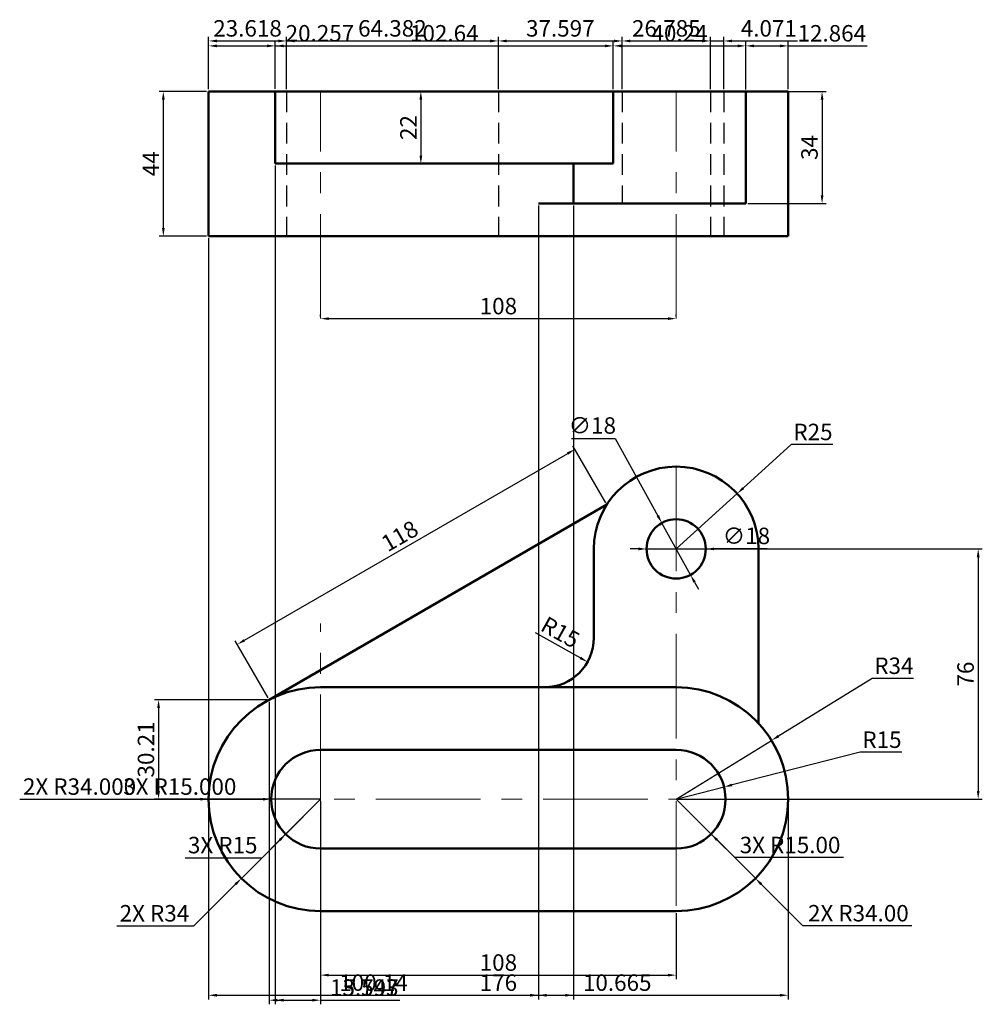
# Model space of a CAD drawing. Units: millimetres. Extents: x 1162 to 1454, y 1698 to 1997.
import ezdxf

# ---------------------------------------------------------------- set-up
doc = ezdxf.new("R2010")
doc.units = ezdxf.units.MM
doc.linetypes.add('CENTER', pattern=[50.8, 31.75, -6.35, 6.35, -6.35])
doc.linetypes.add('HIDDEN', pattern=[9.525, 6.35, -3.175])
for name, color, linetype, lineweight in [('M-CNTR', 1, 'CENTER', 18), ('M-DIMS', 2, 'Continuous', 25), ('M-HIDN', 3, 'HIDDEN', 25), ('M-OUTL', 7, 'Continuous', 50)]:
    doc.layers.add(name, color=color, linetype=linetype, lineweight=lineweight)
doc.styles.get("Standard").update_dxf_attribs({"font": 'arial.ttf'})
doc.dimstyles.new('ISO-25', dxfattribs={"dimtxt": 5, "dimasz": 2.5, "dimexe": 1.25, "dimexo": 0.625, "dimtad": 1, "dimtoh": 1, "dimdec": 0, "dimtxsty": 'Standard', "dimcen": 2.5, "dimadec": 0, "dimazin": 0, "dimtfac": 1, "dimtdec": 0, "dimtmove": 0, "dimatfit": 3, "dimfxl": 1, "dimarcsym": 0})

# ---------------------------------------------------------------- blocks, each defined once
blk = doc.blocks.new('*D1')
at = {"layer": 'Defpoints', "color": 0, "transparency": 16777216}
for p in [(1253.49, 1725.8), (1361.49, 1725.8), (1361.49, 1706.36)]:
    blk.add_point(p, dxfattribs=at)
at = {"layer": 'M-DIMS', "color": 0, "lineweight": -2, "transparency": 16777216}
for p, q in [((1253.49, 1725.18), (1253.49, 1705.11)), ((1361.49, 1725.18), (1361.49, 1705.11)), ((1255.99, 1706.36), (1358.99, 1706.36))]:
    blk.add_line(p, q, dxfattribs=at)
at = {"layer": 'M-DIMS', "color": 0, "transparency": 16777216}
for points in [[(1255.99, 1706.78), (1255.99, 1705.95), (1253.49, 1706.36)], [(1358.99, 1706.78), (1358.99, 1705.95), (1361.49, 1706.36)]]:
    blk.add_solid(points, dxfattribs=at)
at = {"layer": 'M-DIMS', "color": 0, "transparency": 16777216, "insert": (1307.49, 1709.54), "char_height": 5, "attachment_point": 5}
blk.add_mtext('108', dxfattribs=at)
blk = doc.blocks.new('*D2')
at = {"layer": 'Defpoints', "color": 0, "transparency": 16777216}
for p in [(1390.43, 1777.65), (1361.49, 1759.8)]:
    blk.add_point(p, dxfattribs=at)
at = {"layer": 'M-DIMS', "color": 0, "lineweight": -2, "transparency": 16777216}
for p, q in [((1421.01, 1796.5), (1392.56, 1778.96)), ((1433.56, 1796.5), (1421.01, 1796.5)), ((1361.49, 1759.8), (1390.43, 1777.65))]:
    blk.add_line(p, q, dxfattribs=at)
at = {"layer": 'M-DIMS', "color": 0, "transparency": 16777216}
blk.add_solid([(1392.34, 1779.31), (1392.78, 1778.6), (1390.43, 1777.65)], dxfattribs=at)
at = {"layer": 'M-DIMS', "color": 0, "transparency": 16777216, "insert": (1427.6, 1799.68), "char_height": 5, "attachment_point": 5}
blk.add_mtext('R34', dxfattribs=at)
blk = doc.blocks.new('*D3')
at = {"layer": 'Defpoints', "color": 0, "transparency": 16777216}
for p in [(1380, 1852.61), (1361.49, 1835.8)]:
    blk.add_point(p, dxfattribs=at)
at = {"layer": 'M-DIMS', "color": 0, "lineweight": -2, "transparency": 16777216}
for p, q in [((1396.41, 1867.51), (1381.85, 1854.29)), ((1409.02, 1867.51), (1396.41, 1867.51)), ((1361.49, 1835.8), (1380, 1852.61))]:
    blk.add_line(p, q, dxfattribs=at)
at = {"layer": 'M-DIMS', "color": 0, "transparency": 16777216}
blk.add_solid([(1381.57, 1854.6), (1382.13, 1853.98), (1380, 1852.61)], dxfattribs=at)
at = {"layer": 'M-DIMS', "color": 0, "transparency": 16777216, "insert": (1403.03, 1870.69), "char_height": 5, "attachment_point": 5}
blk.add_mtext('R25', dxfattribs=at)
blk = doc.blocks.new('*D4')
at = {"layer": 'Defpoints', "color": 0, "transparency": 16777216}
for p in [(1357.13, 1843.68), (1365.84, 1827.93)]:
    blk.add_point(p, dxfattribs=at)
at = {"layer": 'M-DIMS', "color": 0, "lineweight": -2, "transparency": 16777216}
for p, q in [((1329.71, 1869.33), (1342.95, 1869.33)), ((1342.95, 1869.33), (1355.92, 1845.87)), ((1365.84, 1827.93), (1357.13, 1843.68)), ((1367.05, 1825.74), (1368.26, 1823.55))]:
    blk.add_line(p, q, dxfattribs=at)
at = {"layer": 'M-DIMS', "color": 0, "transparency": 16777216}
for points in [[(1356.29, 1846.07), (1355.56, 1845.67), (1357.13, 1843.68)], [(1367.42, 1825.94), (1366.69, 1825.54), (1365.84, 1827.93)]]:
    blk.add_solid(points, dxfattribs=at)
at = {"layer": 'M-DIMS', "color": 0, "transparency": 16777216, "insert": (1336.02, 1872.65), "char_height": 5, "attachment_point": 5}
blk.add_mtext('∅18', dxfattribs=at)
blk = doc.blocks.new('*D5')
at = {"layer": 'Defpoints', "color": 0, "transparency": 16777216}
for p in [(1376.02, 1763.51), (1361.49, 1759.8)]:
    blk.add_point(p, dxfattribs=at)
at = {"layer": 'M-DIMS', "color": 0, "lineweight": -2, "transparency": 16777216}
for p, q in [((1417.37, 1774.04), (1378.45, 1764.12)), ((1429.98, 1774.04), (1417.37, 1774.04)), ((1361.49, 1759.8), (1376.02, 1763.51))]:
    blk.add_line(p, q, dxfattribs=at)
at = {"layer": 'M-DIMS', "color": 0, "transparency": 16777216}
blk.add_solid([(1378.34, 1764.53), (1378.55, 1763.72), (1376.02, 1763.51)], dxfattribs=at)
at = {"layer": 'M-DIMS', "color": 0, "transparency": 16777216, "insert": (1423.98, 1777.22), "char_height": 5, "attachment_point": 5}
blk.add_mtext('R15', dxfattribs=at)
blk = doc.blocks.new('*D6')
at = {"layer": 'Defpoints', "color": 0, "transparency": 16777216}
for p in [(1321.49, 1808.8), (1334.58, 1801.48)]:
    blk.add_point(p, dxfattribs=at)
at = {"layer": 'M-DIMS', "color": 0, "lineweight": -2, "transparency": 16777216}
blk.add_line((1318.66, 1810.38), (1332.4, 1802.7), dxfattribs=at)
at = {"layer": 'M-DIMS', "color": 0, "transparency": 16777216}
blk.add_solid([(1332.6, 1803.07), (1332.19, 1802.34), (1334.58, 1801.48)], dxfattribs=at)
at = {"layer": 'M-DIMS', "color": 0, "transparency": 16777216, "insert": (1325.99, 1809.93), "char_height": 5, "attachment_point": 5, "rotation": 330.782}
blk.add_mtext('R15', dxfattribs=at)
blk = doc.blocks.new('*D7')
at = {"layer": 'Defpoints', "color": 0, "transparency": 16777216}
for p in [(1330.71, 1866.05), (1340.41, 1849.25), (1237.89, 1790.02)]:
    blk.add_point(p, dxfattribs=at)
at = {"layer": 'M-DIMS', "color": 0, "lineweight": -2, "transparency": 16777216}
for p, q in [((1340.1, 1849.79), (1330.08, 1867.13)), ((1230.35, 1808.06), (1328.54, 1864.8)), ((1237.58, 1790.56), (1227.56, 1807.89))]:
    blk.add_line(p, q, dxfattribs=at)
at = {"layer": 'M-DIMS', "color": 0, "transparency": 16777216}
for points in [[(1328.34, 1865.16), (1328.75, 1864.44), (1330.71, 1866.05)], [(1230.14, 1808.42), (1230.56, 1807.7), (1228.19, 1806.81)]]:
    blk.add_solid(points, dxfattribs=at)
at = {"layer": 'M-DIMS', "color": 0, "transparency": 16777216, "insert": (1277.86, 1839.18), "char_height": 5, "attachment_point": 5, "rotation": 30.0195}
blk.add_mtext('118', dxfattribs=at)
blk = doc.blocks.new('*D8')
at = {"layer": 'Defpoints', "color": 0, "transparency": 16777216}
for p in [(1361.49, 1835.8), (1361.49, 1759.8), (1453.21, 1759.8)]:
    blk.add_point(p, dxfattribs=at)
at = {"layer": 'M-DIMS', "color": 0, "lineweight": -2, "transparency": 16777216}
for p, q in [((1362.11, 1835.8), (1454.46, 1835.8)), ((1453.21, 1833.3), (1453.21, 1762.3)), ((1362.11, 1759.8), (1454.46, 1759.8))]:
    blk.add_line(p, q, dxfattribs=at)
at = {"layer": 'M-DIMS', "color": 0, "transparency": 16777216}
for points in [[(1452.79, 1833.3), (1453.63, 1833.3), (1453.21, 1835.8)], [(1452.79, 1762.3), (1453.63, 1762.3), (1453.21, 1759.8)]]:
    blk.add_solid(points, dxfattribs=at)
at = {"layer": 'M-DIMS', "color": 0, "transparency": 16777216, "insert": (1450.03, 1797.8), "char_height": 5, "attachment_point": 5, "rotation": 90}
blk.add_mtext('76', dxfattribs=at)
blk = doc.blocks.new('*D9')
at = {"layer": 'Defpoints', "color": 0, "transparency": 16777216}
for p in [(1253.49, 1905.75), (1361.49, 1905.75), (1361.49, 1905.75)]:
    blk.add_point(p, dxfattribs=at)
at = {"layer": 'M-DIMS', "color": 0, "lineweight": -2, "transparency": 16777216}
for p, q in [((1253.49, 1906.37), (1253.49, 1907)), ((1255.99, 1905.75), (1358.99, 1905.75)), ((1361.49, 1906.37), (1361.49, 1907))]:
    blk.add_line(p, q, dxfattribs=at)
at = {"layer": 'M-DIMS', "color": 0, "transparency": 16777216}
for points in [[(1255.99, 1906.16), (1255.99, 1905.33), (1253.49, 1905.75)], [(1358.99, 1906.16), (1358.99, 1905.33), (1361.49, 1905.75)]]:
    blk.add_solid(points, dxfattribs=at)
at = {"layer": 'M-DIMS', "color": 0, "transparency": 16777216, "insert": (1307.49, 1908.92), "char_height": 5, "attachment_point": 5}
blk.add_mtext('108', dxfattribs=at)
blk = doc.blocks.new('*D10')
at = {"layer": 'Defpoints', "color": 0, "transparency": 16777216}
for p in [(1219.49, 1974.79), (1205.73, 1930.79), (1219.49, 1930.79)]:
    blk.add_point(p, dxfattribs=at)
at = {"layer": 'M-DIMS', "color": 0, "lineweight": -2, "transparency": 16777216}
for p, q in [((1218.86, 1974.79), (1204.48, 1974.79)), ((1205.73, 1972.29), (1205.73, 1933.29)), ((1218.86, 1930.79), (1204.48, 1930.79))]:
    blk.add_line(p, q, dxfattribs=at)
at = {"layer": 'M-DIMS', "color": 0, "transparency": 16777216}
for points in [[(1205.32, 1972.29), (1206.15, 1972.29), (1205.73, 1974.79)], [(1205.32, 1933.29), (1206.15, 1933.29), (1205.73, 1930.79)]]:
    blk.add_solid(points, dxfattribs=at)
at = {"layer": 'M-DIMS', "color": 0, "transparency": 16777216, "insert": (1202.61, 1952.79), "char_height": 5, "attachment_point": 5, "rotation": 90}
blk.add_mtext('44', dxfattribs=at)
blk = doc.blocks.new('*D11')
at = {"layer": 'Defpoints', "color": 0, "transparency": 16777216}
for p in [(1307.49, 1974.79), (1283.94, 1952.79), (1307.49, 1952.79)]:
    blk.add_point(p, dxfattribs=at)
at = {"layer": 'M-DIMS', "color": 0, "lineweight": -2, "transparency": 16777216}
for p, q in [((1306.86, 1974.79), (1282.69, 1974.79)), ((1283.94, 1972.29), (1283.94, 1955.29)), ((1306.86, 1952.79), (1282.69, 1952.79))]:
    blk.add_line(p, q, dxfattribs=at)
at = {"layer": 'M-DIMS', "color": 0, "transparency": 16777216}
for points in [[(1283.52, 1972.29), (1284.36, 1972.29), (1283.94, 1974.79)], [(1283.52, 1955.29), (1284.36, 1955.29), (1283.94, 1952.79)]]:
    blk.add_solid(points, dxfattribs=at)
at = {"layer": 'M-DIMS', "color": 0, "transparency": 16777216, "insert": (1280.81, 1963.79), "char_height": 5, "attachment_point": 5, "rotation": 90}
blk.add_mtext('22', dxfattribs=at)
blk = doc.blocks.new('*D12')
at = {"layer": 'Defpoints', "color": 0, "transparency": 16777216}
for p in [(1382.62, 1974.73), (1382.62, 1940.73), (1405.8, 1940.73)]:
    blk.add_point(p, dxfattribs=at)
at = {"layer": 'M-DIMS', "color": 0, "lineweight": -2, "transparency": 16777216}
for p, q in [((1383.25, 1974.73), (1407.05, 1974.73)), ((1405.8, 1972.23), (1405.8, 1943.23)), ((1383.25, 1940.73), (1407.05, 1940.73))]:
    blk.add_line(p, q, dxfattribs=at)
at = {"layer": 'M-DIMS', "color": 0, "transparency": 16777216}
for points in [[(1405.38, 1972.23), (1406.22, 1972.23), (1405.8, 1974.73)], [(1405.38, 1943.23), (1406.22, 1943.23), (1405.8, 1940.73)]]:
    blk.add_solid(points, dxfattribs=at)
at = {"layer": 'M-DIMS', "color": 0, "transparency": 16777216, "insert": (1402.62, 1957.73), "char_height": 5, "attachment_point": 5, "rotation": 90}
blk.add_mtext('34', dxfattribs=at)
blk = doc.blocks.new('*D13')
at = {"layer": 'Defpoints', "color": 0, "transparency": 16777216}
for p in [(1239.74, 1988.59), (1219.49, 1974.79), (1239.74, 1974.89)]:
    blk.add_point(p, dxfattribs=at)
at = {"layer": 'M-DIMS', "color": 0, "lineweight": -2, "transparency": 16777216}
for p, q in [((1219.49, 1975.41), (1219.49, 1989.84)), ((1239.74, 1975.51), (1239.74, 1989.84)), ((1221.99, 1988.59), (1237.24, 1988.59)), ((1239.74, 1988.59), (1264.34, 1988.59))]:
    blk.add_line(p, q, dxfattribs=at)
at = {"layer": 'M-DIMS', "color": 0, "transparency": 16777216}
for points in [[(1221.99, 1989), (1221.99, 1988.17), (1219.49, 1988.59)], [(1237.24, 1989), (1237.24, 1988.17), (1239.74, 1988.59)]]:
    blk.add_solid(points, dxfattribs=at)
at = {"layer": 'M-DIMS', "color": 0, "transparency": 16777216, "insert": (1253.29, 1991.77), "char_height": 5, "attachment_point": 5}
blk.add_mtext('20.257', dxfattribs=at)
blk = doc.blocks.new('*D14')
at = {"layer": 'Defpoints', "color": 0, "transparency": 16777216}
for p in [(1342.38, 1988.59), (1239.74, 1974.89), (1342.38, 1974.79)]:
    blk.add_point(p, dxfattribs=at)
at = {"layer": 'M-DIMS', "color": 0, "lineweight": -2, "transparency": 16777216}
for p, q in [((1239.74, 1975.51), (1239.74, 1989.84)), ((1342.38, 1975.41), (1342.38, 1989.84)), ((1242.24, 1988.59), (1339.88, 1988.59))]:
    blk.add_line(p, q, dxfattribs=at)
at = {"layer": 'M-DIMS', "color": 0, "transparency": 16777216}
for points in [[(1242.24, 1989), (1242.24, 1988.17), (1239.74, 1988.59)], [(1339.88, 1989), (1339.88, 1988.17), (1342.38, 1988.59)]]:
    blk.add_solid(points, dxfattribs=at)
at = {"layer": 'M-DIMS', "color": 0, "transparency": 16777216, "insert": (1291.06, 1991.77), "char_height": 5, "attachment_point": 5}
blk.add_mtext('102.64', dxfattribs=at)
blk = doc.blocks.new('*D15')
at = {"layer": 'Defpoints', "color": 0, "transparency": 16777216}
for p in [(1382.62, 1988.59), (1342.38, 1974.79), (1382.62, 1974.73)]:
    blk.add_point(p, dxfattribs=at)
at = {"layer": 'M-DIMS', "color": 0, "lineweight": -2, "transparency": 16777216}
for p, q in [((1342.38, 1975.41), (1342.38, 1989.84)), ((1382.62, 1975.36), (1382.62, 1989.84)), ((1344.88, 1988.59), (1380.12, 1988.59))]:
    blk.add_line(p, q, dxfattribs=at)
at = {"layer": 'M-DIMS', "color": 0, "transparency": 16777216}
for points in [[(1344.88, 1989), (1344.88, 1988.17), (1342.38, 1988.59)], [(1380.12, 1989), (1380.12, 1988.17), (1382.62, 1988.59)]]:
    blk.add_solid(points, dxfattribs=at)
at = {"layer": 'M-DIMS', "color": 0, "transparency": 16777216, "insert": (1362.5, 1991.77), "char_height": 5, "attachment_point": 5}
blk.add_mtext('40.24', dxfattribs=at)
blk = doc.blocks.new('*D16')
at = {"layer": 'Defpoints', "color": 0, "transparency": 16777216}
for p in [(1395.49, 1988.59), (1382.62, 1974.73), (1395.49, 1974.79)]:
    blk.add_point(p, dxfattribs=at)
at = {"layer": 'M-DIMS', "color": 0, "lineweight": -2, "transparency": 16777216}
for p, q in [((1382.62, 1975.36), (1382.62, 1989.84)), ((1395.49, 1975.41), (1395.49, 1989.84)), ((1385.12, 1988.59), (1392.99, 1988.59)), ((1395.49, 1988.59), (1419.5, 1988.59))]:
    blk.add_line(p, q, dxfattribs=at)
at = {"layer": 'M-DIMS', "color": 0, "transparency": 16777216}
for points in [[(1385.12, 1989), (1385.12, 1988.17), (1382.62, 1988.59)], [(1392.99, 1989), (1392.99, 1988.17), (1395.49, 1988.59)]]:
    blk.add_solid(points, dxfattribs=at)
at = {"layer": 'M-DIMS', "color": 0, "transparency": 16777216, "insert": (1408.75, 1991.77), "char_height": 5, "attachment_point": 5}
blk.add_mtext('12.864', dxfattribs=at)
blk = doc.blocks.new('*D17')
at = {"layer": 'Defpoints', "color": 0, "transparency": 16777216}
for p in [(1319.63, 1940.73), (1219.49, 1930.79), (1319.63, 1700.25)]:
    blk.add_point(p, dxfattribs=at)
at = {"layer": 'M-DIMS', "color": 0, "lineweight": -2, "transparency": 16777216}
for p, q in [((1319.63, 1940.11), (1319.63, 1699)), ((1219.49, 1930.16), (1219.49, 1699)), ((1221.99, 1700.25), (1317.13, 1700.25))]:
    blk.add_line(p, q, dxfattribs=at)
at = {"layer": 'M-DIMS', "color": 0, "transparency": 16777216}
for points in [[(1221.99, 1700.67), (1221.99, 1699.83), (1219.49, 1700.25)], [(1317.13, 1700.67), (1317.13, 1699.83), (1319.63, 1700.25)]]:
    blk.add_solid(points, dxfattribs=at)
at = {"layer": 'M-DIMS', "color": 0, "transparency": 16777216, "insert": (1269.56, 1703.43), "char_height": 5, "attachment_point": 5}
blk.add_mtext('100.14', dxfattribs=at)
blk = doc.blocks.new('*D18')
at = {"layer": 'Defpoints', "color": 0, "transparency": 16777216}
for p in [(1319.63, 1940.73), (1330.3, 1940.73), (1330.3, 1700.25)]:
    blk.add_point(p, dxfattribs=at)
at = {"layer": 'M-DIMS', "color": 0, "lineweight": -2, "transparency": 16777216}
for p, q in [((1319.63, 1940.11), (1319.63, 1699)), ((1330.3, 1940.11), (1330.3, 1699)), ((1322.13, 1700.25), (1327.8, 1700.25)), ((1330.3, 1700.25), (1354.37, 1700.25))]:
    blk.add_line(p, q, dxfattribs=at)
at = {"layer": 'M-DIMS', "color": 0, "transparency": 16777216}
for points in [[(1322.13, 1700.67), (1322.13, 1699.83), (1319.63, 1700.25)], [(1327.8, 1700.67), (1327.8, 1699.83), (1330.3, 1700.25)]]:
    blk.add_solid(points, dxfattribs=at)
at = {"layer": 'M-DIMS', "color": 0, "transparency": 16777216, "insert": (1343.58, 1703.43), "char_height": 5, "attachment_point": 5}
blk.add_mtext('10.665', dxfattribs=at)
blk = doc.blocks.new('*D19')
at = {"layer": 'Defpoints', "color": 0, "transparency": 16777216}
for p in [(1219.49, 1759.8), (1395.49, 1759.8), (1395.49, 1700.25)]:
    blk.add_point(p, dxfattribs=at)
at = {"layer": 'M-DIMS', "color": 0, "lineweight": -2, "transparency": 16777216}
for p, q in [((1219.49, 1759.18), (1219.49, 1699)), ((1395.49, 1759.18), (1395.49, 1699)), ((1221.99, 1700.25), (1392.99, 1700.25))]:
    blk.add_line(p, q, dxfattribs=at)
at = {"layer": 'M-DIMS', "color": 0, "transparency": 16777216}
for points in [[(1221.99, 1700.67), (1221.99, 1699.83), (1219.49, 1700.25)], [(1392.99, 1700.67), (1392.99, 1699.83), (1395.49, 1700.25)]]:
    blk.add_solid(points, dxfattribs=at)
at = {"layer": 'M-DIMS', "color": 0, "transparency": 16777216, "insert": (1307.49, 1703.43), "char_height": 5, "attachment_point": 5}
blk.add_mtext('176', dxfattribs=at)
blk = doc.blocks.new('*D20')
at = {"layer": 'Defpoints', "color": 0, "transparency": 16777216}
for p in [(1253.49, 1759.8), (1229.45, 1735.75)]:
    blk.add_point(p, dxfattribs=at)
at = {"layer": 'M-DIMS', "color": 0, "lineweight": -2, "transparency": 16777216}
for p, q in [((1253.49, 1759.8), (1229.45, 1735.75)), ((1215.03, 1721.32), (1227.69, 1733.99)), ((1191.65, 1721.32), (1215.03, 1721.32))]:
    blk.add_line(p, q, dxfattribs=at)
at = {"layer": 'M-DIMS', "color": 0, "transparency": 16777216}
blk.add_solid([(1227.39, 1734.28), (1227.98, 1733.69), (1229.45, 1735.75)], dxfattribs=at)
at = {"layer": 'M-DIMS', "color": 0, "transparency": 16777216, "insert": (1203.03, 1724.5), "char_height": 5, "attachment_point": 5}
blk.add_mtext('2X R34', dxfattribs=at)
blk = doc.blocks.new('*D21')
at = {"layer": 'Defpoints', "color": 0, "transparency": 16777216}
for p in [(1253.49, 1759.8), (1242.89, 1749.19)]:
    blk.add_point(p, dxfattribs=at)
at = {"layer": 'M-DIMS', "color": 0, "lineweight": -2, "transparency": 16777216}
for p, q in [((1253.49, 1759.8), (1242.89, 1749.19)), ((1235.75, 1742.03), (1241.12, 1747.42)), ((1212.4, 1742.03), (1235.75, 1742.03))]:
    blk.add_line(p, q, dxfattribs=at)
at = {"layer": 'M-DIMS', "color": 0, "transparency": 16777216}
blk.add_solid([(1240.83, 1747.71), (1241.42, 1747.13), (1242.89, 1749.19)], dxfattribs=at)
at = {"layer": 'M-DIMS', "color": 0, "transparency": 16777216, "insert": (1223.76, 1745.21), "char_height": 5, "attachment_point": 5}
blk.add_mtext('3X R15', dxfattribs=at)
blk = doc.blocks.new('*D22')
at = {"layer": 'Defpoints', "color": 0, "transparency": 16777216}
for p in [(1352.49, 1835.8), (1370.49, 1835.8)]:
    blk.add_point(p, dxfattribs=at)
at = {"layer": 'M-DIMS', "color": 0, "lineweight": -2, "transparency": 16777216}
for p, q in [((1349.99, 1835.8), (1347.49, 1835.8)), ((1352.49, 1835.8), (1370.49, 1835.8)), ((1375.89, 1835.8), (1372.99, 1835.8)), ((1389.12, 1835.8), (1375.89, 1835.8))]:
    blk.add_line(p, q, dxfattribs=at)
at = {"layer": 'M-DIMS', "color": 0, "transparency": 16777216}
for points in [[(1349.99, 1836.22), (1349.99, 1835.39), (1352.49, 1835.8)], [(1372.99, 1836.22), (1372.99, 1835.39), (1370.49, 1835.8)]]:
    blk.add_solid(points, dxfattribs=at)
at = {"layer": 'M-DIMS', "color": 0, "transparency": 16777216, "insert": (1382.82, 1839.12), "char_height": 5, "attachment_point": 5}
blk.add_mtext('∅18', dxfattribs=at)
blk = doc.blocks.new('*D23')
at = {"layer": 'Defpoints', "color": 0, "transparency": 16777216}
for p in [(1237.89, 1790.02), (1204.29, 1759.8), (1253.49, 1759.8)]:
    blk.add_point(p, dxfattribs=at)
at = {"layer": 'M-DIMS', "color": 0, "lineweight": -2, "transparency": 16777216}
for p, q in [((1237.27, 1790.02), (1203.04, 1790.02)), ((1204.29, 1787.52), (1204.29, 1762.3)), ((1252.86, 1759.8), (1203.04, 1759.8))]:
    blk.add_line(p, q, dxfattribs=at)
at = {"layer": 'M-DIMS', "color": 0, "transparency": 16777216}
for points in [[(1203.87, 1787.52), (1204.7, 1787.52), (1204.29, 1790.02)], [(1203.87, 1762.3), (1204.7, 1762.3), (1204.29, 1759.8)]]:
    blk.add_solid(points, dxfattribs=at)
at = {"layer": 'M-DIMS', "color": 0, "transparency": 16777216, "insert": (1201.11, 1774.91), "char_height": 5, "attachment_point": 5, "rotation": 90}
blk.add_mtext('30.21', dxfattribs=at)
blk = doc.blocks.new('*D24')
at = {"layer": 'Defpoints', "color": 0, "transparency": 16777216}
for p in [(1237.89, 1790.02), (1253.49, 1759.8), (1253.49, 1698.75)]:
    blk.add_point(p, dxfattribs=at)
at = {"layer": 'M-DIMS', "color": 0, "lineweight": -2, "transparency": 16777216}
for p, q in [((1237.89, 1789.39), (1237.89, 1697.5)), ((1253.49, 1759.18), (1253.49, 1697.5)), ((1240.39, 1698.75), (1250.99, 1698.75)), ((1253.49, 1698.75), (1277.52, 1698.75))]:
    blk.add_line(p, q, dxfattribs=at)
at = {"layer": 'M-DIMS', "color": 0, "transparency": 16777216}
for points in [[(1240.39, 1699.17), (1240.39, 1698.33), (1237.89, 1698.75)], [(1250.99, 1699.17), (1250.99, 1698.33), (1253.49, 1698.75)]]:
    blk.add_solid(points, dxfattribs=at)
at = {"layer": 'M-DIMS', "color": 0, "transparency": 16777216, "insert": (1266.76, 1701.93), "char_height": 5, "attachment_point": 5}
blk.add_mtext('15.597', dxfattribs=at)
blk = doc.blocks.new('*D25')
at = {"layer": 'Defpoints', "color": 0, "transparency": 16777216}
for p in [(1239.74, 1952.89), (1253.49, 1759.8), (1253.49, 1698.75)]:
    blk.add_point(p, dxfattribs=at)
at = {"layer": 'M-DIMS', "color": 0, "lineweight": -2, "transparency": 16777216}
for p, q in [((1239.74, 1952.26), (1239.74, 1697.5)), ((1253.49, 1759.18), (1253.49, 1697.5)), ((1242.24, 1698.75), (1250.99, 1698.75)), ((1253.49, 1698.75), (1277.52, 1698.75))]:
    blk.add_line(p, q, dxfattribs=at)
at = {"layer": 'M-DIMS', "color": 0, "transparency": 16777216}
for points in [[(1242.24, 1699.17), (1242.24, 1698.33), (1239.74, 1698.75)], [(1250.99, 1699.17), (1250.99, 1698.33), (1253.49, 1698.75)]]:
    blk.add_solid(points, dxfattribs=at)
at = {"layer": 'M-DIMS', "color": 0, "transparency": 16777216, "insert": (1266.76, 1701.93), "char_height": 5, "attachment_point": 5}
blk.add_mtext('13.743', dxfattribs=at)
blk = doc.blocks.new('*D26')
at = {"layer": 'Defpoints', "color": 0, "transparency": 16777216}
for p in [(1361.49, 1759.8), (1385.53, 1735.77)]:
    blk.add_point(p, dxfattribs=at)
at = {"layer": 'M-DIMS', "color": 0, "lineweight": -2, "transparency": 16777216}
for p, q in [((1361.49, 1759.8), (1385.53, 1735.77)), ((1399.96, 1721.34), (1387.3, 1734)), ((1433.06, 1721.34), (1399.96, 1721.34))]:
    blk.add_line(p, q, dxfattribs=at)
at = {"layer": 'M-DIMS', "color": 0, "transparency": 16777216}
blk.add_solid([(1387.6, 1734.29), (1387.01, 1733.7), (1385.53, 1735.77)], dxfattribs=at)
at = {"layer": 'M-DIMS', "color": 0, "transparency": 16777216, "insert": (1416.82, 1724.52), "char_height": 5, "attachment_point": 5}
blk.add_mtext('2X R34.00', dxfattribs=at)
blk = doc.blocks.new('*D27')
at = {"layer": 'Defpoints', "color": 0, "transparency": 16777216}
for p in [(1361.49, 1759.8), (1372.1, 1749.2)]:
    blk.add_point(p, dxfattribs=at)
at = {"layer": 'M-DIMS', "color": 0, "lineweight": -2, "transparency": 16777216}
for p, q in [((1361.49, 1759.8), (1372.1, 1749.2)), ((1379.25, 1742.06), (1373.87, 1747.43)), ((1412.26, 1742.06), (1379.25, 1742.06))]:
    blk.add_line(p, q, dxfattribs=at)
at = {"layer": 'M-DIMS', "color": 0, "transparency": 16777216}
blk.add_solid([(1374.16, 1747.73), (1373.57, 1747.14), (1372.1, 1749.2)], dxfattribs=at)
at = {"layer": 'M-DIMS', "color": 0, "transparency": 16777216, "insert": (1396.07, 1745.24), "char_height": 5, "attachment_point": 5}
blk.add_mtext('3X R15.00', dxfattribs=at)
blk = doc.blocks.new('*D28')
at = {"layer": 'Defpoints', "color": 0, "transparency": 16777216}
for p in [(1243.11, 1990.09), (1219.49, 1974.79), (1243.11, 1974.79)]:
    blk.add_point(p, dxfattribs=at)
at = {"layer": 'M-DIMS', "color": 0, "lineweight": -2, "transparency": 16777216}
for p, q in [((1219.49, 1975.41), (1219.49, 1991.34)), ((1221.99, 1990.09), (1240.61, 1990.09)), ((1243.11, 1975.41), (1243.11, 1991.34))]:
    blk.add_line(p, q, dxfattribs=at)
at = {"layer": 'M-DIMS', "color": 0, "transparency": 16777216}
for points in [[(1221.99, 1990.5), (1221.99, 1989.67), (1219.49, 1990.09)], [(1240.61, 1990.5), (1240.61, 1989.67), (1243.11, 1990.09)]]:
    blk.add_solid(points, dxfattribs=at)
at = {"layer": 'M-DIMS', "color": 0, "transparency": 16777216, "insert": (1231.3, 1993.27), "char_height": 5, "attachment_point": 5}
blk.add_mtext('23.618', dxfattribs=at)
blk = doc.blocks.new('*D29')
at = {"layer": 'Defpoints', "color": 0, "transparency": 16777216}
for p in [(1307.49, 1990.09), (1243.11, 1974.79), (1307.49, 1974.79)]:
    blk.add_point(p, dxfattribs=at)
at = {"layer": 'M-DIMS', "color": 0, "lineweight": -2, "transparency": 16777216}
for p, q in [((1243.11, 1975.41), (1243.11, 1991.34)), ((1245.61, 1990.09), (1304.99, 1990.09)), ((1307.49, 1975.41), (1307.49, 1991.34))]:
    blk.add_line(p, q, dxfattribs=at)
at = {"layer": 'M-DIMS', "color": 0, "transparency": 16777216}
for points in [[(1245.61, 1990.5), (1245.61, 1989.67), (1243.11, 1990.09)], [(1304.99, 1990.5), (1304.99, 1989.67), (1307.49, 1990.09)]]:
    blk.add_solid(points, dxfattribs=at)
at = {"layer": 'M-DIMS', "color": 0, "transparency": 16777216, "insert": (1275.3, 1993.27), "char_height": 5, "attachment_point": 5}
blk.add_mtext('64.382', dxfattribs=at)
blk = doc.blocks.new('*D30')
at = {"layer": 'Defpoints', "color": 0, "transparency": 16777216}
for p in [(1345.08, 1990.09), (1307.49, 1974.79), (1345.08, 1974.79)]:
    blk.add_point(p, dxfattribs=at)
at = {"layer": 'M-DIMS', "color": 0, "lineweight": -2, "transparency": 16777216}
for p, q in [((1307.49, 1975.41), (1307.49, 1991.34)), ((1309.99, 1990.09), (1342.58, 1990.09)), ((1345.08, 1975.41), (1345.08, 1991.34))]:
    blk.add_line(p, q, dxfattribs=at)
at = {"layer": 'M-DIMS', "color": 0, "transparency": 16777216}
for points in [[(1309.99, 1990.5), (1309.99, 1989.67), (1307.49, 1990.09)], [(1342.58, 1990.5), (1342.58, 1989.67), (1345.08, 1990.09)]]:
    blk.add_solid(points, dxfattribs=at)
at = {"layer": 'M-DIMS', "color": 0, "transparency": 16777216, "insert": (1326.29, 1993.27), "char_height": 5, "attachment_point": 5}
blk.add_mtext('37.597', dxfattribs=at)
blk = doc.blocks.new('*D31')
at = {"layer": 'Defpoints', "color": 0, "transparency": 16777216}
for p in [(1371.87, 1990.09), (1345.08, 1974.79), (1371.87, 1974.79)]:
    blk.add_point(p, dxfattribs=at)
at = {"layer": 'M-DIMS', "color": 0, "lineweight": -2, "transparency": 16777216}
for p, q in [((1345.08, 1975.41), (1345.08, 1991.34)), ((1347.58, 1990.09), (1369.37, 1990.09)), ((1371.87, 1975.41), (1371.87, 1991.34))]:
    blk.add_line(p, q, dxfattribs=at)
at = {"layer": 'M-DIMS', "color": 0, "transparency": 16777216}
for points in [[(1347.58, 1990.5), (1347.58, 1989.67), (1345.08, 1990.09)], [(1369.37, 1990.5), (1369.37, 1989.67), (1371.87, 1990.09)]]:
    blk.add_solid(points, dxfattribs=at)
at = {"layer": 'M-DIMS', "color": 0, "transparency": 16777216, "insert": (1358.48, 1993.27), "char_height": 5, "attachment_point": 5}
blk.add_mtext('26.785', dxfattribs=at)
blk = doc.blocks.new('*D32')
at = {"layer": 'Defpoints', "color": 0, "transparency": 16777216}
for p in [(1375.94, 1990.09), (1371.87, 1974.79), (1375.94, 1974.79)]:
    blk.add_point(p, dxfattribs=at)
at = {"layer": 'M-DIMS', "color": 0, "lineweight": -2, "transparency": 16777216}
for p, q in [((1369.37, 1990.09), (1366.87, 1990.09)), ((1371.87, 1975.41), (1371.87, 1991.34)), ((1371.87, 1990.09), (1375.94, 1990.09)), ((1375.94, 1975.41), (1375.94, 1991.34)), ((1378.44, 1990.09), (1398.3, 1990.09))]:
    blk.add_line(p, q, dxfattribs=at)
at = {"layer": 'M-DIMS', "color": 0, "transparency": 16777216}
for points in [[(1369.37, 1990.5), (1369.37, 1989.67), (1371.87, 1990.09)], [(1378.44, 1990.5), (1378.44, 1989.67), (1375.94, 1990.09)]]:
    blk.add_solid(points, dxfattribs=at)
at = {"layer": 'M-DIMS', "color": 0, "transparency": 16777216, "insert": (1389.62, 1993.27), "char_height": 5, "attachment_point": 5}
blk.add_mtext('4.071', dxfattribs=at)
blk = doc.blocks.new('*D33')
at = {"layer": 'Defpoints', "color": 0, "transparency": 16777216}
for p in [(1219.49, 1759.8), (1253.49, 1759.8)]:
    blk.add_point(p, dxfattribs=at)
at = {"layer": 'M-DIMS', "color": 0, "lineweight": -2, "transparency": 16777216}
for p, q in [((1162.11, 1759.8), (1199.09, 1759.8)), ((1199.09, 1759.8), (1216.99, 1759.8)), ((1253.49, 1759.8), (1219.49, 1759.8))]:
    blk.add_line(p, q, dxfattribs=at)
at = {"layer": 'M-DIMS', "color": 0, "transparency": 16777216}
blk.add_solid([(1216.99, 1760.22), (1216.99, 1759.39), (1219.49, 1759.8)], dxfattribs=at)
at = {"layer": 'M-DIMS', "color": 0, "transparency": 16777216, "insert": (1180.29, 1762.98), "char_height": 5, "attachment_point": 5}
blk.add_mtext('2X R34.000', dxfattribs=at)
blk = doc.blocks.new('*D34')
at = {"layer": 'Defpoints', "color": 0, "transparency": 16777216}
for p in [(1238.49, 1759.8), (1253.49, 1759.8)]:
    blk.add_point(p, dxfattribs=at)
at = {"layer": 'M-DIMS', "color": 0, "lineweight": -2, "transparency": 16777216}
for p, q in [((1192.6, 1759.8), (1229.49, 1759.8)), ((1229.49, 1759.8), (1235.99, 1759.8)), ((1253.49, 1759.8), (1238.49, 1759.8))]:
    blk.add_line(p, q, dxfattribs=at)
at = {"layer": 'M-DIMS', "color": 0, "transparency": 16777216}
blk.add_solid([(1235.99, 1760.22), (1235.99, 1759.39), (1238.49, 1759.8)], dxfattribs=at)
at = {"layer": 'M-DIMS', "color": 0, "transparency": 16777216, "insert": (1210.73, 1762.98), "char_height": 5, "attachment_point": 5}
blk.add_mtext('3X R15.000', dxfattribs=at)

msp = doc.modelspace()

# ---------------------------------------------------------------- linework, layer by layer
at = {"layer": 'M-CNTR'}
for p, q in [((1253.4872, 1905.7464), (1253.4872, 1974.7868)), ((1361.4872, 1905.7464), (1361.4872, 1974.7868)), ((1361.4872, 1860.8035), (1361.4872, 1714.1546)), ((1253.4872, 1759.8035), (1253.4872, 1813.1897)), ((1219.4872, 1759.8035), (1395.4872, 1759.8035)), ((1253.4872, 1759.8035), (1253.4872, 1713.951))]:
    msp.add_line(p, q, dxfattribs=at)
at = {"layer": 'M-HIDN'}
for p, q in [((1243.105, 1974.7868), (1243.105, 1930.7868)), ((1243.105, 1974.7868), (1243.105, 1930.7868)), ((1243.105, 1974.7868), (1243.105, 1930.7868)), ((1307.4872, 1974.7868), (1307.4872, 1930.7868)), ((1345.0839, 1974.7868), (1345.0839, 1940.7321)), ((1371.8693, 1974.7868), (1371.8693, 1930.7868)), ((1375.94, 1974.7868), (1375.94, 1930.7868))]:
    msp.add_line(p, q, dxfattribs=at)
at = {"layer": 'M-OUTL'}
for p, q in [((1395.4872, 1974.7868), (1219.4872, 1974.7868)), ((1219.4872, 1974.7868), (1219.4872, 1930.7868)), ((1239.7445, 1974.8883), (1239.7445, 1952.8883)), ((1342.3807, 1952.8883), (1342.3807, 1974.7868)), ((1382.6231, 1974.7321), (1382.6231, 1940.7321)), ((1395.4872, 1930.7868), (1395.4872, 1974.7868)), ((1239.7445, 1952.8883), (1342.3807, 1952.8883)), ((1330.2957, 1940.7321), (1330.2957, 1952.8883)), ((1382.6231, 1940.7321), (1319.6312, 1940.7321)), ((1219.4872, 1930.7868), (1395.4872, 1930.7868)), ((1237.8905, 1790.0151), (1340.4134, 1849.2532)), ((1336.4872, 1835.8035), (1336.4872, 1808.8035)), ((1386.4872, 1835.8035), (1386.4872, 1782.8469)), ((1253.4872, 1793.8035), (1321.4872, 1793.8035)), ((1321.4872, 1793.8035), (1361.4872, 1793.8035)), ((1253.4872, 1774.8035), (1361.4872, 1774.8035)), ((1361.4872, 1744.8035), (1253.4872, 1744.8035)), ((1253.4872, 1725.8035), (1361.4872, 1725.8035))]:
    msp.add_line(p, q, dxfattribs=at)
msp.add_circle((1361.4872, 1835.8035), 9, dxfattribs=at)
for centre, radius, start, end in [((1361.4872, 1835.8035), 25, 0, 180), ((1321.4872, 1808.8035), 15, 270, 0), ((1253.4872, 1759.8035), 34, 90, 270), ((1361.4872, 1759.8035), 34, 270, 90), ((1253.4872, 1759.8035), 15, 90, 270), ((1361.4872, 1759.8035), 15, 270, 90)]:
    msp.add_arc(centre, radius, start, end, dxfattribs=at)

# ---------------------------------------------------------------- dimensions: what is measured, and where the dimension line sits
at = {"layer": 'M-DIMS'}
for base, p1, p2, override, picture, middle in [((1243.105, 1990.0883), (1219.4872, 1974.7868), (1243.105, 1974.7868), {"dimdec": 3, "dimlfac": 1, "dimrnd": 0, "dimzin": 0, "dimdsep": 46, "dimlunit": 2}, '*D28', (1231.2961, 1993.2679)), ((1239.7445, 1988.5883), (1219.4872, 1974.7868), (1239.7445, 1974.8883), {"dimdec": 3, "dimlfac": 1, "dimrnd": 0, "dimzin": 0, "dimdsep": 46, "dimlunit": 2}, '*D13', (1253.2908, 1991.7662)), ((1342.3807, 1988.5883), (1239.7445, 1974.8883), (1342.3807, 1974.7868), {"dimdec": 2, "dimlfac": 1, "dimrnd": 0, "dimzin": 0, "dimdsep": 46, "dimlunit": 2}, '*D14', (1291.0626, 1991.7662)), ((1307.4872, 1990.0883), (1243.105, 1974.7868), (1307.4872, 1974.7868), {"dimdec": 3, "dimlfac": 1, "dimrnd": 0, "dimzin": 0, "dimdsep": 46, "dimlunit": 2}, '*D29', (1275.2961, 1993.2679)), ((1345.0839, 1990.0883), (1307.4872, 1974.7868), (1345.0839, 1974.7868), {"dimdec": 3, "dimlfac": 1, "dimrnd": 0, "dimzin": 0, "dimdsep": 46, "dimlunit": 2}, '*D30', (1326.2855, 1993.2679)), ((1382.6231, 1988.5883), (1342.3807, 1974.7868), (1382.6231, 1974.7321), {"dimdec": 2, "dimlfac": 1, "dimrnd": 0, "dimzin": 0, "dimdsep": 46, "dimlunit": 2}, '*D15', (1362.5019, 1991.7662)), ((1371.8693, 1990.0883), (1345.0839, 1974.7868), (1371.8693, 1974.7868), {"dimdec": 3, "dimlfac": 1, "dimrnd": 0, "dimzin": 0, "dimdsep": 46, "dimlunit": 2}, '*D31', (1358.4766, 1993.2662)), ((1375.94, 1990.0883), (1371.8693, 1974.7868), (1375.94, 1974.7868), {"dimdec": 3, "dimlfac": 1, "dimrnd": 0, "dimzin": 0, "dimdsep": 46, "dimlunit": 2}, '*D32', (1389.6192, 1993.2662)), ((1395.4872, 1988.5883), (1382.6231, 1974.7321), (1395.4872, 1974.7868), {"dimdec": 3, "dimlfac": 1, "dimrnd": 0, "dimzin": 0, "dimdsep": 46, "dimlunit": 2}, '*D16', (1408.7452, 1991.7662)), ((1253.4872, 1698.751), (1239.7445, 1952.8883), (1253.4872, 1759.8035), {"dimdec": 3, "dimlfac": 1, "dimrnd": 0, "dimzin": 0, "dimdsep": 46, "dimlunit": 2}, '*D25', (1266.7554, 1701.9305)), ((1319.6312, 1700.251), (1219.4872, 1930.7868), (1319.6312, 1940.7321), {"dimdec": 2, "dimlfac": 1, "dimrnd": 0, "dimzin": 0, "dimdsep": 46, "dimlunit": 2}, '*D17', (1269.5592, 1703.4288)), ((1330.29571, 1700.25096), (1319.63117, 1940.73214), (1330.29571, 1940.73214), {"dimdec": 3, "dimlfac": 1, "dimrnd": 0, "dimzin": 0, "dimdsep": 46, "dimlunit": 2}, '*D18', (1343.58272, 1703.42882)), ((1361.4872, 1905.7464), (1253.4872, 1905.7464), (1361.4872, 1905.7464), {"dimclrd": 0, "dimclre": 0, "dimclrt": 0}, '*D9', (1307.4872, 1908.9242)), ((1253.4872, 1698.751), (1237.8905, 1790.0151), (1253.4872, 1759.8035), {"dimdec": 3, "dimlfac": 1, "dimrnd": 0, "dimzin": 0, "dimdsep": 46, "dimlunit": 2}, '*D24', (1266.7554, 1701.9288)), ((1395.4872, 1700.251), (1219.4872, 1759.8035), (1395.4872, 1759.8035), {"dimdec": 0, "dimlfac": 1, "dimrnd": 0, "dimzin": 0, "dimdsep": 46, "dimlunit": 2}, '*D19', (1307.4872, 1703.4288)), ((1361.4872, 1706.3639), (1253.4872, 1725.8035), (1361.4872, 1725.8035), {"dimclrd": 0, "dimclre": 0, "dimclrt": 0}, '*D1', (1307.4872, 1709.5418))]:
    dim = msp.add_linear_dim(base=base, p1=p1, p2=p2, dimstyle='ISO-25', override=override, dxfattribs=at)
    dim.commit()
    dim.dimension.update_dxf_attribs({"geometry": picture, "text_midpoint": middle})
for base, p1, p2, override, picture, middle in [((1205.7337, 1930.7868), (1219.4872, 1974.7868), (1219.4872, 1930.7868), {"dimclrd": 0, "dimclre": 0, "dimclrt": 0}, '*D10', (1202.6087, 1952.7868)), ((1283.9404, 1952.7868), (1307.4872, 1974.7868), (1307.4872, 1952.7868), {"dimclrd": 0, "dimclre": 0, "dimclrt": 0}, '*D11', (1280.8052, 1963.7868)), ((1405.8008, 1940.7321), (1382.6231, 1974.7321), (1382.6231, 1940.7321), {"dimclrd": 0, "dimclre": 0, "dimclrt": 0}, '*D12', (1402.6212, 1957.7321)), ((1453.209, 1759.8035), (1361.4872, 1835.8035), (1361.4872, 1759.8035), {"dimclrd": 0, "dimclre": 0, "dimclrt": 0}, '*D8', (1450.0311, 1797.8035)), ((1204.2872, 1759.8035), (1237.8905, 1790.0151), (1253.4872, 1759.8035), {"dimdec": 2, "dimlfac": 1, "dimrnd": 0, "dimzin": 0, "dimdsep": 46, "dimlunit": 2}, '*D23', (1201.1076, 1774.9093))]:
    dim = msp.add_linear_dim(base=base, p1=p1, p2=p2, angle=90, dimstyle='ISO-25', override=override, dxfattribs=at)
    dim.commit()
    dim.dimension.update_dxf_attribs({"geometry": picture, "text_midpoint": middle})
for p1, p2, override, picture, middle in [((1365.8419, 1827.9272), (1357.1324, 1843.6798), {"dimclrd": 0, "dimclre": 0, "dimclrt": 0}, '*D4', (1336.0171, 1869.334)), ((1352.4872, 1835.803), (1370.4872, 1835.804), {"dimdec": 0, "dimlfac": 1, "dimrnd": 0, "dimzin": 0, "dimdsep": 46, "dimlunit": 2}, '*D22', (1375.8872, 1835.8043))]:
    dim = msp.add_diameter_dim_2p(p1=p1, p2=p2, dimstyle='ISO-25', override=override, dxfattribs=at)
    dim.commit()
    dim.dimension.update_dxf_attribs({"geometry": picture, "text_midpoint": middle, "dimtype": 163})
for center, mpoint, picture, middle in [((1361.4872, 1835.8035), (1379.9953, 1852.6097), '*D3', (1403.0255, 1867.5131)), ((1321.4872, 1808.8035), (1334.5787, 1801.4815), '*D6', (1324.4393, 1807.1524)), ((1361.4872, 1759.8035), (1390.4296, 1777.6455), '*D2', (1427.6002, 1796.4982)), ((1361.4872, 1759.8035), (1376.0228, 1763.5069), '*D5', (1417.3667, 1774.0405))]:
    dim = msp.add_radius_dim(center=center, mpoint=mpoint, dimstyle='ISO-25', override={"dimclrd": 0, "dimclre": 0, "dimclrt": 0}, dxfattribs=at)
    dim.commit()
    dim.dimension.update_dxf_attribs({"geometry": picture, "text_midpoint": middle, "dimtype": 164})
dim = msp.add_aligned_dim(p1=(1237.8905, 1790.0151), p2=(1340.4134, 1849.2532), distance=19.3988, dimstyle='ISO-25', override={"dimclrd": 0, "dimclre": 0, "dimclrt": 0}, dxfattribs=at)
dim.commit()
dim.dimension.update_dxf_attribs({"geometry": '*D7', "text_midpoint": (1277.857, 1839.1823)})
for center, mpoint, text, override, picture, middle in [((1253.4872, 1759.8035), (1219.4872, 1759.804), '2X <>', {"dimdec": 3, "dimlfac": 1, "dimrnd": 0, "dimzin": 0, "dimdsep": 46, "dimlunit": 2}, '*D33', (1199.0872, 1759.8043)), ((1253.4872, 1759.8035), (1238.4872, 1759.804), '3X <>', {"dimdec": 3, "dimlfac": 1, "dimrnd": 0, "dimzin": 0, "dimdsep": 46, "dimlunit": 2}, '*D34', (1229.4872, 1759.8043)), ((1253.4872, 1759.8035), (1229.4537, 1735.7537), '2X <>', {"dimdec": 0, "dimlfac": 1, "dimrnd": 0, "dimzin": 0, "dimdsep": 46, "dimlunit": 2}, '*D20', (1203.0308, 1721.3238)), ((1361.4872, 1759.8035), (1385.5335, 1735.7665), '2X <>', {"dimdec": 2, "dimlfac": 1, "dimrnd": 0, "dimzin": 0, "dimdsep": 46, "dimlunit": 2}, '*D26', (1416.8209, 1721.3444))]:
    dim = msp.add_radius_dim(center=center, mpoint=mpoint, text=text, dimstyle='ISO-25', override=override, dxfattribs=at)
    dim.commit()
    dim.dimension.update_dxf_attribs({"geometry": picture, "text_midpoint": middle, "dimtype": 164})
for center, mpoint, override, picture, middle in [((1253.4872, 1759.8035), (1242.8887, 1749.1887), {"dimdec": 0, "dimlfac": 1, "dimrnd": 0, "dimzin": 0, "dimdsep": 46, "dimlunit": 2}, '*D21', (1223.7585, 1745.2145)), ((1361.4872, 1759.8035), (1372.0984, 1749.2016), {"dimdec": 2, "dimlfac": 1, "dimrnd": 0, "dimzin": 0, "dimdsep": 46, "dimlunit": 2}, '*D27', (1396.0651, 1745.236))]:
    dim = msp.add_radius_dim(center=center, mpoint=mpoint, text='3X <>', dimstyle='ISO-25', override=override, dxfattribs=at)
    dim.commit()
    dim.dimension.update_dxf_attribs({"geometry": picture, "text_midpoint": middle})

doc.saveas('drawing.dxf')
